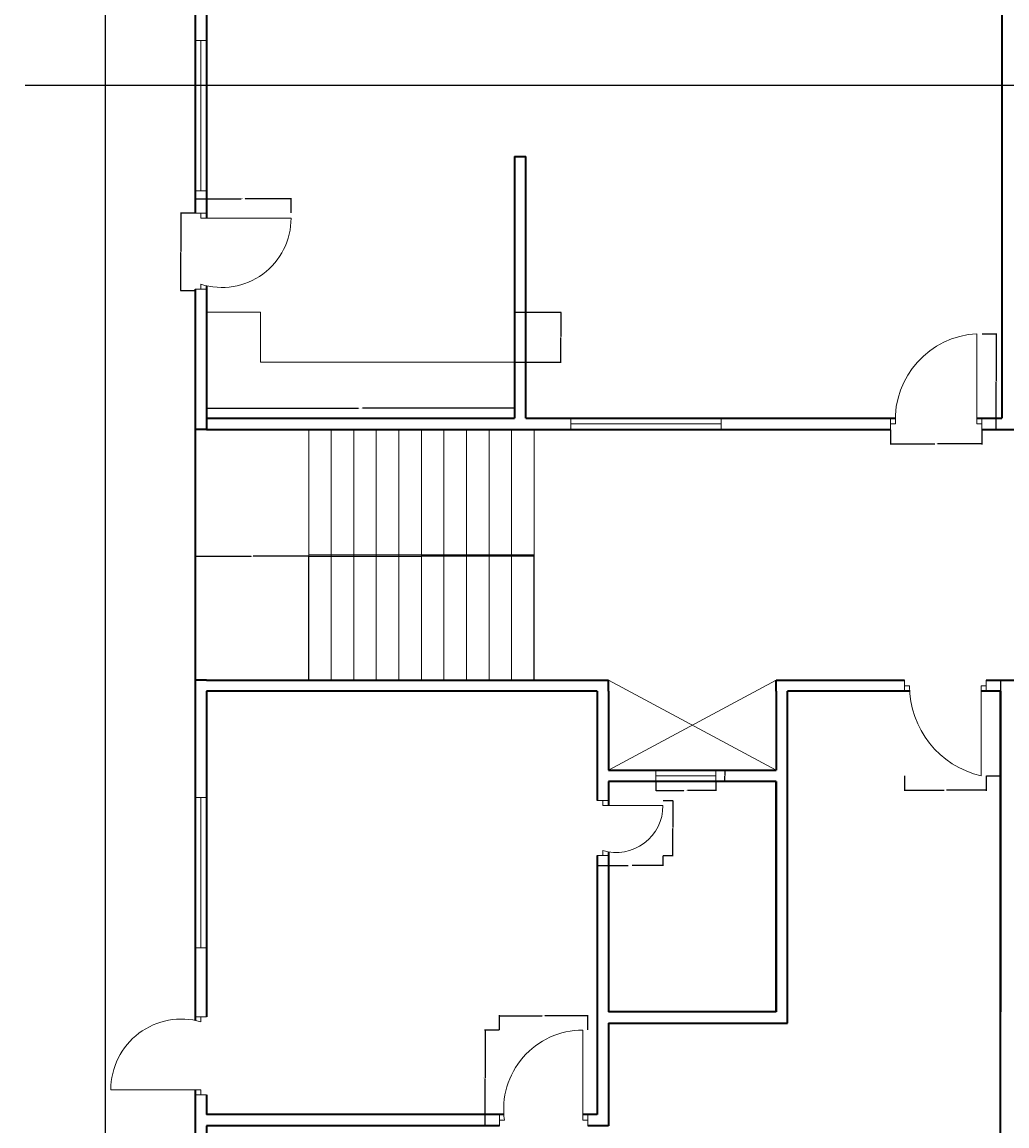
# Model space of a CAD drawing. Units: inches. Extents: x 1520 to 3401, y 1570 to 3432.
# Tile 11 of 15: x 2435 to 2828, y 2061 to 2501. Entities that reach past the tile are written whole.
import ezdxf

# ---------------------------------------------------------------- set-up
doc = ezdxf.new("R2010")
doc.units = ezdxf.units.IN
for name, color, linetype, lineweight in [('A-ANNO-DIMS', 2, 'Continuous', 18), ('A-ANNO-SYMB', 2, 'Continuous', 25), ('A-DOOR', 3, 'Continuous', 18), ('A-FLOR-CASE', 8, 'Continuous', 18), ('A-FLOR-EDGE', 7, 'Continuous', 25), ('A-FLOR-OPEN', 8, 'Continuous', 13), ('A-FLOR-STRS', 2, 'Continuous', 18), ('A-GLAZ', 4, 'Continuous', 18), ('A-WALL', 7, 'Continuous', 35)]:
    doc.layers.add(name, color=color, linetype=linetype, lineweight=lineweight)
doc.styles.get("Standard").update_dxf_attribs({"font": 'arial.ttf'})
doc.dimstyles.get("Standard").update_dxf_attribs({"dimtxt": 0.18, "dimasz": 0.18, "dimexe": 0.18, "dimexo": 0.0625, "dimgap": 0.09, "dimtad": 0, "dimtih": 1, "dimtoh": 1, "dimdec": 4, "dimzin": 0, "dimdsep": 46, "dimtxsty": 'Standard', "dimcen": 0.09, "dimadec": 0, "dimazin": 0, "dimtfac": 1, "dimtdec": 4, "dimtofl": 0, "dimtmove": 0, "dimatfit": 3, "dimfxl": 1, "dimtolj": 1, "dimtzin": 0, "dimarcsym": 0})

# ---------------------------------------------------------------- blocks, each defined once
blk = doc.blocks.new('DOOR-SWING-36-09')
for p, q in [((34.55, 2.25), (34.55, 38.25)), ((0, 4.5), (0, 0)), ((36.55, 4.5), (36.55, 0)), ((0, 0), (0, 2.25)), ((0, 2.25), (2, 2.25)), ((36.55, 2.25), (34.55, 2.25)), ((36.55, 0), (36.55, 2.25))]:
    blk.add_line(p, q)
blk.add_arc((36.37, 3.88), 34.41, 93.0408, 182.7237)
blk = doc.blocks.new('DOOR-SWING-24-14')
for p, q in [((4.5, 21.95), (0, 21.95)), ((0, 21.95), (2.25, 21.95)), ((2.25, 21.95), (2.25, 19.95)), ((2.25, 19.95), (26.25, 19.95)), ((4.5, 0), (0, 0)), ((0, 0), (2.25, 0)), ((2.25, 0), (2.25, 2))]:
    blk.add_line(p, q)
blk.add_arc((7.54, 19.95), 18.71, 253.5847, 0)
blk = doc.blocks.new('DOOR-SWING-36-15')
for p, q in [((33.3, 2.25), (33.3, 38.25)), ((0, 4.5), (0, 0)), ((35.3, 4.5), (35.3, 0)), ((0, 0), (0, 2.25)), ((0, 2.25), (2, 2.25)), ((35.3, 2.25), (33.3, 2.25)), ((35.3, 0), (35.3, 2.25))]:
    blk.add_line(p, q)
blk.add_arc((33.3, 6.65), 31.6, 90, 187.995)
blk = doc.blocks.new('DOOR-SWING-36-17')
for p, q in [((0, 33.75), (0, 38.25)), ((0, 38.25), (0, 36)), ((0, 36), (2, 36)), ((32.63, 36), (30.63, 36)), ((30.63, 36), (30.63, 0)), ((32.63, 33.75), (32.63, 38.25)), ((32.63, 38.25), (32.63, 36))]:
    blk.add_line(p, q)
blk.add_arc((38.95, 36), 36.95, 180, 256.9796)
blk = doc.blocks.new('DOOR-SWING-36-24')
for p, q in [((0, 30.42), (4.5, 30.42)), ((4.5, 30.42), (2.25, 30.42)), ((2.25, 30.42), (2.25, 28.42)), ((2.25, 28.42), (38.25, 28.42)), ((4.5, 0), (0, 0)), ((0, 0), (2.25, 0)), ((2.25, 0), (2.25, 2))]:
    blk.add_line(p, q)
blk.add_arc((10.55, 28.42), 27.7, 252.5577, 0)
blk = doc.blocks.new('DOOR-SWING-36-25')
for p, q in [((33.75, 31.15), (38.25, 31.15)), ((38.25, 31.15), (36, 31.15)), ((36, 31.15), (36, 29.15)), ((36, 2), (0, 2)), ((38.25, 0), (33.75, 0)), ((33.75, 0), (36, 0)), ((36, 0), (36, 2))]:
    blk.add_line(p, q)
blk.add_arc((28.23, 2), 28.23, 74.0345, 180)
blk = doc.blocks.new('WIN-PLAN-24-01')
for p, q in [((0, 4.5), (0, 0)), ((24, 2.25), (24, 4.5)), ((24, 4.5), (24, 0)), ((0, 0), (0, 2.25)), ((0, 2.25), (24, 2.25))]:
    blk.add_line(p, q)
blk = doc.blocks.new('WIN-PLAN-60-02')
for p, q in [((4.5, 60), (0, 60)), ((0, 60), (2.25, 60)), ((2.25, 60), (2.25, 0)), ((4.5, 0), (0, 0)), ((2.25, 0), (4.5, 0))]:
    blk.add_line(p, q)
blk = doc.blocks.new('WIN-PLAN-60-03')
for p, q in [((0, 2.25), (0, 4.5)), ((0, 4.5), (0, 0)), ((60, 0), (60, 4.5)), ((60, 4.5), (60, 2.25)), ((60, 2.25), (0, 2.25))]:
    blk.add_line(p, q)
blk = doc.blocks.new('KITCHEN-COUNTER-04')
for p, q in [((0, 19.94), (21.46, 19.94)), ((21.46, 19.94), (21.46, 0)), ((21.46, 0), (123, 0)), ((123, 0), (123, 0))]:
    blk.add_line(p, q)
blk = doc.blocks.new('*D63')
at = {"layer": 'A-ANNO-DIMS', "color": 0, "lineweight": -2, "transparency": 16777216}
for p, q in [((2687.73, 2198.12), (2687.73, 2194.4)), ((2687.91, 2194.58), (2698.98, 2194.58)), ((2711.55, 2194.58), (2700.49, 2194.58)), ((2711.73, 2198.12), (2711.73, 2194.4))]:
    blk.add_line(p, q, dxfattribs=at)
at = {"layer": 'A-ANNO-DIMS', "color": 0, "transparency": 16777216}
for points in [[(2687.91, 2194.61), (2687.91, 2194.55), (2687.73, 2194.58)], [(2711.55, 2194.61), (2711.55, 2194.55), (2711.73, 2194.58)]]:
    blk.add_solid(points, dxfattribs=at)
at = {"layer": 'Defpoints', "color": 0, "transparency": 16777216}
for p in [(2687.73, 2198.18), (2711.73, 2198.18), (2711.73, 2194.58)]:
    blk.add_point(p, dxfattribs=at)
at = {"layer": 'A-ANNO-DIMS', "color": 0, "transparency": 16777216, "insert": (2699.73, 2194.58), "char_height": 0.18, "attachment_point": 5}
blk.add_mtext('\\A1;W1 24 TYP.', dxfattribs=at)
blk = doc.blocks.new('*D64')
at = {"layer": 'A-ANNO-DIMS', "color": 0, "lineweight": -2, "transparency": 16777216}
for p, q in [((2711.79, 2202.68), (2715.51, 2202.68)), ((2715.33, 2202.5), (2715.33, 2200.61)), ((2715.33, 2198.36), (2715.33, 2200.25)), ((2711.79, 2198.18), (2715.51, 2198.18))]:
    blk.add_line(p, q, dxfattribs=at)
at = {"layer": 'A-ANNO-DIMS', "color": 0, "transparency": 16777216}
for points in [[(2715.3, 2202.5), (2715.36, 2202.5), (2715.33, 2202.68)], [(2715.3, 2198.36), (2715.36, 2198.36), (2715.33, 2198.18)]]:
    blk.add_solid(points, dxfattribs=at)
at = {"layer": 'Defpoints', "color": 0, "transparency": 16777216}
for p in [(2711.73, 2202.68), (2715.33, 2202.68), (2711.73, 2198.18)]:
    blk.add_point(p, dxfattribs=at)
at = {"layer": 'A-ANNO-DIMS', "color": 0, "transparency": 16777216, "insert": (2715.33, 2200.43), "char_height": 0.18, "attachment_point": 5}
blk.add_mtext('\\A1;5 TYP.', dxfattribs=at)
blk = doc.blocks.new('*D97')
at = {"layer": 'A-ANNO-DIMS', "color": 0, "lineweight": -2, "transparency": 16777216}
for p, q in [((2818.06, 2376.93), (2823.92, 2376.93)), ((2823.74, 2376.75), (2823.74, 2357.99)), ((2823.74, 2338.86), (2823.74, 2357.62)), ((2818.06, 2338.68), (2823.92, 2338.68))]:
    blk.add_line(p, q, dxfattribs=at)
at = {"layer": 'A-ANNO-DIMS', "color": 0, "transparency": 16777216}
for points in [[(2823.71, 2376.75), (2823.77, 2376.75), (2823.74, 2376.93)], [(2823.71, 2338.86), (2823.77, 2338.86), (2823.74, 2338.68)]]:
    blk.add_solid(points, dxfattribs=at)
at = {"layer": 'Defpoints', "color": 0, "transparency": 16777216}
for p in [(2818, 2376.93), (2823.74, 2376.93), (2818, 2338.68)]:
    blk.add_point(p, dxfattribs=at)
at = {"layer": 'A-ANNO-DIMS', "color": 0, "transparency": 16777216, "insert": (2823.74, 2357.8), "char_height": 0.18, "attachment_point": 5}
blk.add_mtext('\\A1;D09 38 TYP.', dxfattribs=at)
blk = doc.blocks.new('*D98')
at = {"layer": 'A-ANNO-DIMS', "color": 0, "lineweight": -2, "transparency": 16777216}
for p, q in [((2781.45, 2338.62), (2781.45, 2332.76)), ((2818, 2338.62), (2818, 2332.76)), ((2781.63, 2332.94), (2799.2, 2332.94)), ((2817.82, 2332.94), (2800.25, 2332.94))]:
    blk.add_line(p, q, dxfattribs=at)
at = {"layer": 'A-ANNO-DIMS', "color": 0, "transparency": 16777216}
for points in [[(2781.63, 2332.97), (2781.63, 2332.91), (2781.45, 2332.94)], [(2817.82, 2332.97), (2817.82, 2332.91), (2818, 2332.94)]]:
    blk.add_solid(points, dxfattribs=at)
at = {"layer": 'Defpoints', "color": 0, "transparency": 16777216}
for p in [(2781.45, 2338.68), (2818, 2338.68), (2818, 2332.94)]:
    blk.add_point(p, dxfattribs=at)
at = {"layer": 'A-ANNO-DIMS', "color": 0, "transparency": 16777216, "insert": (2799.72, 2332.94), "char_height": 0.18, "attachment_point": 5}
blk.add_mtext('\\A1;37 TYP.', dxfattribs=at)
blk = doc.blocks.new('*D107')
at = {"layer": 'A-ANNO-DIMS', "color": 0, "lineweight": -2, "transparency": 16777216}
for p, q in [((2664.4, 2168.53), (2664.4, 2164.47)), ((2690.65, 2168.53), (2690.65, 2164.47)), ((2664.58, 2164.65), (2676.73, 2164.65)), ((2690.47, 2164.65), (2678.31, 2164.65))]:
    blk.add_line(p, q, dxfattribs=at)
at = {"layer": 'A-ANNO-DIMS', "color": 0, "transparency": 16777216}
for points in [[(2664.58, 2164.68), (2664.58, 2164.62), (2664.4, 2164.65)], [(2690.47, 2164.68), (2690.47, 2164.62), (2690.65, 2164.65)]]:
    blk.add_solid(points, dxfattribs=at)
at = {"layer": 'Defpoints', "color": 0, "transparency": 16777216}
for p in [(2664.4, 2168.59), (2690.65, 2168.59), (2690.65, 2164.65)]:
    blk.add_point(p, dxfattribs=at)
at = {"layer": 'A-ANNO-DIMS', "color": 0, "transparency": 16777216, "insert": (2677.52, 2164.65), "char_height": 0.18, "attachment_point": 5}
blk.add_mtext('\\A1;D14 26 TYP.', dxfattribs=at)
blk = doc.blocks.new('*D108')
at = {"layer": 'A-ANNO-DIMS', "color": 0, "lineweight": -2, "transparency": 16777216}
for p, q in [((2690.71, 2190.54), (2694.77, 2190.54)), ((2694.59, 2190.36), (2694.59, 2179.75)), ((2694.59, 2168.77), (2694.59, 2179.39)), ((2690.71, 2168.59), (2694.77, 2168.59))]:
    blk.add_line(p, q, dxfattribs=at)
at = {"layer": 'A-ANNO-DIMS', "color": 0, "transparency": 16777216}
for points in [[(2694.56, 2190.36), (2694.62, 2190.36), (2694.59, 2190.54)], [(2694.56, 2168.77), (2694.62, 2168.77), (2694.59, 2168.59)]]:
    blk.add_solid(points, dxfattribs=at)
at = {"layer": 'Defpoints', "color": 0, "transparency": 16777216}
for p in [(2690.65, 2190.54), (2694.59, 2190.54), (2690.65, 2168.59)]:
    blk.add_point(p, dxfattribs=at)
at = {"layer": 'A-ANNO-DIMS', "color": 0, "transparency": 16777216, "insert": (2694.59, 2179.57), "char_height": 0.18, "attachment_point": 5}
blk.add_mtext('\\A1;22 TYP.', dxfattribs=at)
blk = doc.blocks.new('*D109')
at = {"layer": 'A-ANNO-DIMS', "color": 0, "lineweight": -2, "transparency": 16777216}
for p, q in [((2625.26, 2098.93), (2619.41, 2098.93)), ((2619.59, 2098.75), (2619.59, 2079.99)), ((2619.59, 2060.86), (2619.59, 2079.62)), ((2625.26, 2060.68), (2619.41, 2060.68))]:
    blk.add_line(p, q, dxfattribs=at)
at = {"layer": 'A-ANNO-DIMS', "color": 0, "transparency": 16777216}
for points in [[(2619.56, 2098.75), (2619.62, 2098.75), (2619.59, 2098.93)], [(2619.56, 2060.86), (2619.62, 2060.86), (2619.59, 2060.68)]]:
    blk.add_solid(points, dxfattribs=at)
at = {"layer": 'Defpoints', "color": 0, "transparency": 16777216}
for p in [(2619.59, 2098.93), (2625.32, 2098.93), (2625.32, 2060.68)]:
    blk.add_point(p, dxfattribs=at)
at = {"layer": 'A-ANNO-DIMS', "color": 0, "transparency": 16777216, "insert": (2619.59, 2079.8), "char_height": 0.18, "attachment_point": 5}
blk.add_mtext('\\A1;D15 38 TYP.', dxfattribs=at)
blk = doc.blocks.new('*D110')
at = {"layer": 'A-ANNO-DIMS', "color": 0, "lineweight": -2, "transparency": 16777216}
for p, q in [((2625.32, 2098.99), (2625.32, 2104.85)), ((2625.5, 2104.67), (2642.45, 2104.67)), ((2660.44, 2104.67), (2643.5, 2104.67)), ((2660.62, 2098.99), (2660.62, 2104.85))]:
    blk.add_line(p, q, dxfattribs=at)
at = {"layer": 'A-ANNO-DIMS', "color": 0, "transparency": 16777216}
for points in [[(2625.5, 2104.7), (2625.5, 2104.64), (2625.32, 2104.67)], [(2660.44, 2104.7), (2660.44, 2104.64), (2660.62, 2104.67)]]:
    blk.add_solid(points, dxfattribs=at)
at = {"layer": 'Defpoints', "color": 0, "transparency": 16777216}
for p in [(2660.62, 2104.67), (2625.32, 2098.93), (2660.62, 2098.93)]:
    blk.add_point(p, dxfattribs=at)
at = {"layer": 'A-ANNO-DIMS', "color": 0, "transparency": 16777216, "insert": (2642.97, 2104.67), "char_height": 0.18, "attachment_point": 5}
blk.add_mtext('\\A1;35 TYP.', dxfattribs=at)
blk = doc.blocks.new('*D113')
at = {"layer": 'A-ANNO-DIMS', "color": 0, "lineweight": -2, "transparency": 16777216}
for p, q in [((2819.78, 2238.68), (2825.63, 2238.68)), ((2825.45, 2238.5), (2825.45, 2219.74)), ((2825.45, 2200.61), (2825.45, 2219.37)), ((2819.78, 2200.43), (2825.63, 2200.43))]:
    blk.add_line(p, q, dxfattribs=at)
at = {"layer": 'A-ANNO-DIMS', "color": 0, "transparency": 16777216}
for points in [[(2825.42, 2238.5), (2825.48, 2238.5), (2825.45, 2238.68)], [(2825.42, 2200.61), (2825.48, 2200.61), (2825.45, 2200.43)]]:
    blk.add_solid(points, dxfattribs=at)
at = {"layer": 'Defpoints', "color": 0, "transparency": 16777216}
for p in [(2819.71, 2238.68), (2825.45, 2238.68), (2819.71, 2200.43)]:
    blk.add_point(p, dxfattribs=at)
at = {"layer": 'A-ANNO-DIMS', "color": 0, "transparency": 16777216, "insert": (2825.45, 2219.55), "char_height": 0.18, "attachment_point": 5}
blk.add_mtext('\\A1;D17 38 TYP.', dxfattribs=at)
blk = doc.blocks.new('*D114')
at = {"layer": 'A-ANNO-DIMS', "color": 0, "lineweight": -2, "transparency": 16777216}
for p, q in [((2787.09, 2200.37), (2787.09, 2194.51)), ((2819.71, 2200.37), (2819.71, 2194.51)), ((2787.27, 2194.69), (2802.87, 2194.69)), ((2819.53, 2194.69), (2803.93, 2194.69))]:
    blk.add_line(p, q, dxfattribs=at)
at = {"layer": 'A-ANNO-DIMS', "color": 0, "transparency": 16777216}
for points in [[(2787.27, 2194.72), (2787.27, 2194.66), (2787.09, 2194.69)], [(2819.53, 2194.72), (2819.53, 2194.66), (2819.71, 2194.69)]]:
    blk.add_solid(points, dxfattribs=at)
at = {"layer": 'Defpoints', "color": 0, "transparency": 16777216}
for p in [(2787.09, 2200.43), (2819.71, 2200.43), (2819.71, 2194.69)]:
    blk.add_point(p, dxfattribs=at)
at = {"layer": 'A-ANNO-DIMS', "color": 0, "transparency": 16777216, "insert": (2803.4, 2194.69), "char_height": 0.18, "attachment_point": 5}
blk.add_mtext('\\A1;33 TYP.', dxfattribs=at)
blk = doc.blocks.new('*D127')
at = {"layer": 'A-ANNO-DIMS', "color": 0, "lineweight": -2, "transparency": 16777216}
for p, q in [((2503.9, 2425.16), (2503.9, 2431.02)), ((2504.08, 2430.84), (2522.23, 2430.84)), ((2541.97, 2430.84), (2523.81, 2430.84)), ((2542.15, 2425.16), (2542.15, 2431.02))]:
    blk.add_line(p, q, dxfattribs=at)
at = {"layer": 'A-ANNO-DIMS', "color": 0, "transparency": 16777216}
for points in [[(2504.08, 2430.87), (2504.08, 2430.81), (2503.9, 2430.84)], [(2541.97, 2430.87), (2541.97, 2430.81), (2542.15, 2430.84)]]:
    blk.add_solid(points, dxfattribs=at)
at = {"layer": 'Defpoints', "color": 0, "transparency": 16777216}
for p in [(2542.15, 2430.84), (2503.9, 2425.1), (2542.15, 2425.1)]:
    blk.add_point(p, dxfattribs=at)
at = {"layer": 'A-ANNO-DIMS', "color": 0, "transparency": 16777216, "insert": (2523.02, 2430.84), "char_height": 0.18, "attachment_point": 5}
blk.add_mtext('\\A1;D24 38 TYP.', dxfattribs=at)
blk = doc.blocks.new('*D128')
at = {"layer": 'A-ANNO-DIMS', "color": 0, "lineweight": -2, "transparency": 16777216}
for p, q in [((2503.84, 2425.1), (2497.98, 2425.1)), ((2498.16, 2424.92), (2498.16, 2409.75)), ((2498.16, 2394.21), (2498.16, 2409.38)), ((2503.84, 2394.03), (2497.98, 2394.03))]:
    blk.add_line(p, q, dxfattribs=at)
at = {"layer": 'A-ANNO-DIMS', "color": 0, "transparency": 16777216}
for points in [[(2498.13, 2424.92), (2498.19, 2424.92), (2498.16, 2425.1)], [(2498.13, 2394.21), (2498.19, 2394.21), (2498.16, 2394.03)]]:
    blk.add_solid(points, dxfattribs=at)
at = {"layer": 'Defpoints', "color": 0, "transparency": 16777216}
for p in [(2498.16, 2425.1), (2503.9, 2425.1), (2503.9, 2394.03)]:
    blk.add_point(p, dxfattribs=at)
at = {"layer": 'A-ANNO-DIMS', "color": 0, "transparency": 16777216, "insert": (2498.16, 2409.56), "char_height": 0.18, "attachment_point": 5}
blk.add_mtext('\\A1;31 TYP.', dxfattribs=at)
blk = doc.blocks.new('*D155')
at = {"layer": 'A-ANNO-DIMS', "color": 0, "lineweight": -2, "transparency": 16777216}
for p, q in [((2508.4, 2365.57), (2508.4, 2347)), ((2631.4, 2365.57), (2631.4, 2347)), ((2508.58, 2347.18), (2569.11, 2347.18)), ((2631.22, 2347.18), (2570.69, 2347.18))]:
    blk.add_line(p, q, dxfattribs=at)
at = {"layer": 'A-ANNO-DIMS', "color": 0, "transparency": 16777216}
for points in [[(2508.58, 2347.21), (2508.58, 2347.15), (2508.4, 2347.18)], [(2631.22, 2347.21), (2631.22, 2347.15), (2631.4, 2347.18)]]:
    blk.add_solid(points, dxfattribs=at)
at = {"layer": 'Defpoints', "color": 0, "transparency": 16777216}
for p in [(2508.4, 2365.63), (2631.4, 2365.63), (2631.4, 2347.18)]:
    blk.add_point(p, dxfattribs=at)
at = {"layer": 'A-ANNO-DIMS', "color": 0, "transparency": 16777216, "insert": (2569.9, 2347.18), "char_height": 0.18, "attachment_point": 5}
blk.add_mtext('\\A1;C4 123 TYP.', dxfattribs=at)
blk = doc.blocks.new('*D156')
at = {"layer": 'A-ANNO-DIMS', "color": 0, "lineweight": -2, "transparency": 16777216}
for p, q in [((2631.46, 2385.57), (2650.03, 2385.57)), ((2649.85, 2385.39), (2649.85, 2375.78)), ((2649.85, 2365.81), (2649.85, 2375.42)), ((2631.46, 2365.63), (2650.03, 2365.63))]:
    blk.add_line(p, q, dxfattribs=at)
at = {"layer": 'A-ANNO-DIMS', "color": 0, "transparency": 16777216}
for points in [[(2649.82, 2385.39), (2649.88, 2385.39), (2649.85, 2385.57)], [(2649.82, 2365.81), (2649.88, 2365.81), (2649.85, 2365.63)]]:
    blk.add_solid(points, dxfattribs=at)
at = {"layer": 'Defpoints', "color": 0, "transparency": 16777216}
for p in [(2631.4, 2385.57), (2649.85, 2385.57), (2631.4, 2365.63)]:
    blk.add_point(p, dxfattribs=at)
at = {"layer": 'A-ANNO-DIMS', "color": 0, "transparency": 16777216, "insert": (2649.85, 2375.6), "char_height": 0.18, "attachment_point": 5}
blk.add_mtext('\\A1;20 TYP.', dxfattribs=at)
blk = doc.blocks.new('*D192')
at = {"layer": 'A-ANNO-DIMS', "color": 0, "lineweight": -2, "transparency": 16777216}
for p, q in [((2467.84, 2733.18), (2386.32, 2733.18)), ((2386.5, 2733), (2386.5, 2244.61)), ((2386.5, 1755.86), (2386.5, 2244.25)), ((2503.84, 1755.68), (2386.32, 1755.68))]:
    blk.add_line(p, q, dxfattribs=at)
at = {"layer": 'A-ANNO-DIMS', "color": 0, "transparency": 16777216}
for points in [[(2386.47, 2733), (2386.53, 2733), (2386.5, 2733.18)], [(2386.47, 1755.86), (2386.53, 1755.86), (2386.5, 1755.68)]]:
    blk.add_solid(points, dxfattribs=at)
at = {"layer": 'Defpoints', "color": 0, "transparency": 16777216}
for p in [(2467.9, 2733.18), (2386.5, 1755.68), (2503.9, 1755.68)]:
    blk.add_point(p, dxfattribs=at)
at = {"layer": 'A-ANNO-DIMS', "color": 0, "transparency": 16777216, "insert": (2386.5, 2244.43), "char_height": 0.18, "attachment_point": 5}
blk.add_mtext('\\A1;977.5', dxfattribs=at)
blk = doc.blocks.new('*D207')
at = {"layer": 'A-ANNO-DIMS', "color": 0, "lineweight": -2, "transparency": 16777216}
for p, q in [((2549.18, 2238.74), (2549.18, 2288.26)), ((2549.36, 2288.08), (2593.96, 2288.08)), ((2639, 2288.08), (2594.4, 2288.08)), ((2639.18, 2238.74), (2639.18, 2288.26))]:
    blk.add_line(p, q, dxfattribs=at)
at = {"layer": 'A-ANNO-DIMS', "color": 0, "transparency": 16777216}
for points in [[(2549.36, 2288.11), (2549.36, 2288.05), (2549.18, 2288.08)], [(2639, 2288.11), (2639, 2288.05), (2639.18, 2288.08)]]:
    blk.add_solid(points, dxfattribs=at)
at = {"layer": 'Defpoints', "color": 0, "transparency": 16777216}
for p in [(2639.18, 2288.08), (2549.18, 2238.68), (2639.18, 2238.68)]:
    blk.add_point(p, dxfattribs=at)
at = {"layer": 'A-ANNO-DIMS', "color": 0, "transparency": 16777216, "insert": (2594.18, 2288.08), "char_height": 0.18, "attachment_point": 5}
blk.add_mtext('\\A1;90', dxfattribs=at)
blk = doc.blocks.new('*D208')
at = {"layer": 'A-ANNO-DIMS', "color": 0, "lineweight": -2, "transparency": 16777216}
for p, q in [((2503.9, 2238.74), (2503.9, 2288.26)), ((2504.08, 2288.08), (2526.14, 2288.08)), ((2549, 2288.08), (2526.94, 2288.08)), ((2549.18, 2238.74), (2549.18, 2288.26))]:
    blk.add_line(p, q, dxfattribs=at)
at = {"layer": 'A-ANNO-DIMS', "color": 0, "transparency": 16777216}
for points in [[(2504.08, 2288.11), (2504.08, 2288.05), (2503.9, 2288.08)], [(2549, 2288.11), (2549, 2288.05), (2549.18, 2288.08)]]:
    blk.add_solid(points, dxfattribs=at)
at = {"layer": 'Defpoints', "color": 0, "transparency": 16777216}
for p in [(2549.18, 2288.08), (2503.9, 2238.68), (2549.18, 2238.68)]:
    blk.add_point(p, dxfattribs=at)
at = {"layer": 'A-ANNO-DIMS', "color": 0, "transparency": 16777216, "insert": (2526.54, 2288.08), "char_height": 0.18, "attachment_point": 5}
blk.add_mtext('\\A1;45.28', dxfattribs=at)

msp = doc.modelspace()

# ---------------------------------------------------------------- linework, layer by layer
at = {"layer": 'A-ANNO-SYMB'}
msp.add_line((2435.8982, 2476.123), (3251.5148, 2476.123), dxfattribs=at)
at = {"layer": 'A-FLOR-EDGE'}
msp.add_line((2467.8987, 2733.1786), (2467.8987, 1791.6786), dxfattribs=at)
at = {"layer": 'A-FLOR-OPEN'}
for p, q in [((2735.8987, 2238.6786), (2668.8987, 2202.6786)), ((2668.8987, 2238.6786), (2735.8987, 2202.6786))]:
    msp.add_line(p, q, dxfattribs=at)
at = {"layer": 'A-FLOR-STRS'}
for p, q in [((2549.1766, 2238.6786), (2549.1766, 2338.6786)), ((2549.1766, 2338.6786), (2549.1766, 2288.6786)), ((2558.1766, 2238.6786), (2558.1766, 2338.6786)), ((2558.1766, 2338.6786), (2558.1766, 2288.6786)), ((2567.1766, 2238.6786), (2567.1766, 2338.6786)), ((2567.1766, 2338.6786), (2567.1766, 2288.6786)), ((2576.1766, 2238.6786), (2576.1766, 2338.6786)), ((2576.1766, 2338.6786), (2576.1766, 2288.6786)), ((2585.1766, 2238.6786), (2585.1766, 2338.6786)), ((2585.1766, 2338.6786), (2585.1766, 2288.6786)), ((2594.1766, 2238.6786), (2594.1766, 2338.6786)), ((2594.1766, 2338.6786), (2594.1766, 2288.6786)), ((2603.1766, 2238.6786), (2603.1766, 2338.6786)), ((2603.1766, 2338.6786), (2603.1766, 2288.6786)), ((2612.1766, 2238.6786), (2612.1766, 2338.6786)), ((2612.1766, 2338.6786), (2612.1766, 2288.6786)), ((2621.1766, 2238.6786), (2621.1766, 2338.6786)), ((2621.1766, 2338.6786), (2621.1766, 2288.6786)), ((2630.1766, 2238.6786), (2630.1766, 2338.6786)), ((2630.1766, 2338.6786), (2630.1766, 2288.6786)), ((2639.1766, 2238.6786), (2639.1766, 2338.6786)), ((2549.1766, 2288.6786), (2639.1766, 2288.6786))]:
    msp.add_line(p, q, dxfattribs=at)
at = {"layer": 'A-WALL'}
for p, q in [((2825.8987, 2558.1786), (2825.8987, 2343.1786)), ((2503.8987, 2508.6786), (2503.8987, 2425.0977)), ((2503.8987, 2508.6786), (2503.8987, 2425.0977)), ((2508.3987, 2508.6786), (2508.3987, 2423.0977)), ((2631.3987, 2447.697), (2631.3987, 2343.1786)), ((2631.3987, 2447.697), (2635.8987, 2447.697)), ((2635.8987, 2343.1786), (2635.8987, 2447.697)), ((2503.8987, 2394.6735), (2503.8987, 2102.8094)), ((2503.8987, 2394.6735), (2503.8987, 2102.8094)), ((2508.3987, 2396.0692), (2508.3987, 2338.6786)), ((2508.3987, 2343.1786), (2631.3987, 2343.1786)), ((2635.8987, 2343.1786), (2783.4164, 2343.1786)), ((2815.9986, 2343.1786), (2825.8987, 2343.1786)), ((2508.3987, 2338.6786), (2503.8987, 2338.6786)), ((2508.3987, 2338.6786), (2781.4498, 2338.6786)), ((2817.9986, 2338.6786), (2967.3389, 2338.6786)), ((2508.3987, 2238.6786), (2503.8987, 2238.6786)), ((2508.3987, 2238.6786), (2668.8987, 2238.6786)), ((2668.8987, 2234.1786), (2668.8987, 2238.6786)), ((2735.8987, 2238.6786), (2787.088, 2238.6786)), ((2735.8987, 2234.1786), (2735.8987, 2238.6786)), ((2819.7132, 2238.6786), (3032.072, 2238.6786)), ((2508.3987, 2234.1786), (2508.3987, 2104.2644)), ((2664.3987, 2234.1786), (2508.3987, 2234.1786)), ((2664.3987, 2234.1786), (2664.3987, 2190.5406)), ((2668.8987, 2234.1786), (2668.8987, 2202.6786)), ((2735.8987, 2234.1786), (2735.8987, 2202.6786)), ((2789.1566, 2234.1786), (2740.3987, 2234.1786)), ((2740.3987, 2106.1786), (2740.3987, 2234.1786)), ((2825.3987, 2234.1786), (2817.7132, 2234.1786)), ((2825.3987, 1923.6786), (2825.3987, 2234.1786)), ((2825.3987, 2234.1786), (2825.3987, 2106.1786)), ((2668.8987, 2202.6786), (2735.8987, 2202.6786)), ((2668.8987, 2198.1786), (2668.8987, 2188.5406)), ((2735.8987, 2198.1786), (2668.8987, 2198.1786)), ((2735.8987, 2198.1786), (2735.8987, 2106.1786)), ((2735.8987, 2106.1786), (2735.8987, 2198.1786)), ((2664.3987, 2168.5913), (2664.3987, 2065.1786)), ((2668.8987, 2170.0769), (2668.8987, 2106.1786)), ((2735.8987, 2106.1786), (2668.8987, 2106.1786)), ((2740.3987, 2101.6786), (2740.3987, 2106.1786)), ((2668.8987, 2101.6786), (2668.8987, 2060.6786)), ((2668.8987, 2101.6786), (2740.3987, 2101.6786)), ((2503.8987, 2075.1195), (2503.8987, 1924.1968)), ((2503.8987, 2075.1195), (2503.8987, 1924.1968)), ((2508.3987, 2073.1195), (2508.3987, 2065.1786)), ((2627.0907, 2065.1786), (2508.3987, 2065.1786)), ((2664.3987, 2065.1786), (2658.622, 2065.1786)), ((2508.3987, 2060.6786), (2508.3987, 1922.1968)), ((2625.3249, 2060.6786), (2508.3987, 2060.6786)), ((2668.8987, 2060.6786), (2660.622, 2060.6786))]:
    msp.add_line(p, q, dxfattribs=at)

# ---------------------------------------------------------------- block references
at = {"layer": 'A-DOOR'}
for name, p in [('DOOR-SWING-36-24', (2503.8988, 2394.673)), ('DOOR-SWING-36-09', (2781.4498, 2338.679)), ('DOOR-SWING-36-17', (2787.0878, 2200.429)), ('DOOR-SWING-24-14', (2664.3988, 2168.591)), ('DOOR-SWING-36-25', (2470.1488, 2073.119)), ('DOOR-SWING-36-15', (2625.3248, 2060.679))]:
    msp.add_blockref(name, p, dxfattribs=at)
at = {"layer": 'A-FLOR-CASE'}
msp.add_blockref('KITCHEN-COUNTER-04', (2508.3988, 2365.63), dxfattribs=at)
at = {"layer": 'A-GLAZ', "extrusion": (0, 0, -1), "zscale": -1, "rotation": 90}
msp.add_blockref('WIN-PLAN-60-03', (-2503.899, 2434.0305), dxfattribs=at)
at = {"layer": 'A-GLAZ'}
for name, p, rotation in [('WIN-PLAN-60-02', (2653.8695, 2343.1785), 270), ('WIN-PLAN-60-03', (2508.3983, 2131.8338), 90)]:
    msp.add_blockref(name, p, dxfattribs=dict(at, rotation=rotation))
msp.add_blockref('WIN-PLAN-24-01', (2687.7318, 2198.179), dxfattribs=at)

# ---------------------------------------------------------------- dimensions: what is measured, and where the dimension line sits
at = {"layer": 'A-ANNO-DIMS'}
dim = msp.add_linear_dim(base=(2386.4982, 1755.6786), p1=(2467.8987, 2733.1786), p2=(2503.8987, 1755.6786), angle=90, dimstyle='Standard', override={"dimdec": 1, "dimlfac": 1, "dimrnd": 0, "dimzin": 0, "dimdsep": 46, "dimlunit": 2}, dxfattribs=at)
dim.commit()
dim.dimension.update_dxf_attribs({"geometry": '*D192', "text_midpoint": (2386.4982, 2244.4286)})
for base, p1, p2, text, picture, middle in [((2542.1487, 2430.8352), (2503.8987, 2425.0977), (2542.1487, 2425.0977), 'D24 <> TYP.', '*D127', (2523.0237, 2430.8352)), ((2631.3987, 2347.1795), (2508.3987, 2365.6295), (2631.3987, 2365.6295), 'C4 <> TYP.', '*D155', (2569.8987, 2347.1795)), ((2817.9986, 2332.9411), (2781.4498, 2338.6786), (2817.9986, 2338.6786), '<> TYP.', '*D98', (2799.7242, 2332.9411)), ((2819.7132, 2194.6911), (2787.088, 2200.4286), (2819.7132, 2200.4286), '<> TYP.', '*D114', (2803.4006, 2194.6911)), ((2711.7322, 2194.5786), (2687.7322, 2198.1786), (2711.7322, 2198.1786), 'W1 <> TYP.', '*D63', (2699.7322, 2194.5786)), ((2690.6487, 2164.6538), (2664.3987, 2168.5913), (2690.6487, 2168.5913), 'D14 <> TYP.', '*D107', (2677.5237, 2164.6538)), ((2660.622, 2104.6661), (2625.3249, 2098.9286), (2660.622, 2098.9286), '<> TYP.', '*D110', (2642.9735, 2104.6661))]:
    dim = msp.add_linear_dim(base=base, p1=p1, p2=p2, text=text, dimstyle='Standard', override={"dimdec": 0, "dimlfac": 1, "dimrnd": 0, "dimzin": 0, "dimdsep": 46, "dimlunit": 2}, dxfattribs=at)
    dim.commit()
    dim.dimension.update_dxf_attribs({"geometry": picture, "text_midpoint": middle})
for base, p1, p2, text, picture, middle in [((2498.1612, 2425.0977), (2503.8987, 2394.0301), (2503.8987, 2425.0977), '<> TYP.', '*D128', (2498.1612, 2409.5639)), ((2649.8487, 2385.5713), (2631.3987, 2365.6295), (2631.3987, 2385.5713), '<> TYP.', '*D156', (2649.8487, 2375.6004)), ((2823.7361, 2376.9286), (2817.9986, 2338.6786), (2817.9986, 2376.9286), 'D09 <> TYP.', '*D97', (2823.7361, 2357.8036)), ((2825.4507, 2238.6786), (2819.7132, 2200.4286), (2819.7132, 2238.6786), 'D17 <> TYP.', '*D113', (2825.4507, 2219.5536)), ((2715.3321503742, 2202.6786294992), (2711.7321503742, 2198.1786294992), (2711.7321503742, 2202.6786294992), '<> TYP.', '*D64', (2715.3321503742, 2200.4286294992)), ((2694.5862, 2190.5406), (2690.6487, 2168.5913), (2690.6487, 2190.5406), '<> TYP.', '*D108', (2694.5862, 2179.566)), ((2619.5874, 2098.9286), (2625.3249, 2060.6786), (2625.3249, 2098.9286), 'D15 <> TYP.', '*D109', (2619.5874, 2079.8036))]:
    dim = msp.add_linear_dim(base=base, p1=p1, p2=p2, angle=90, text=text, dimstyle='Standard', override={"dimdec": 0, "dimlfac": 1, "dimrnd": 0, "dimzin": 0, "dimdsep": 46, "dimlunit": 2}, dxfattribs=at)
    dim.commit()
    dim.dimension.update_dxf_attribs({"geometry": picture, "text_midpoint": middle})
for base, p1, p2, override, picture, middle in [((2549.1766, 2288.0786), (2503.8987, 2238.6786), (2549.1766, 2238.6786), {"dimdec": 2, "dimlfac": 1, "dimrnd": 0, "dimzin": 0, "dimdsep": 46, "dimlunit": 2}, '*D208', (2526.5376, 2288.0786)), ((2639.1766, 2288.0786), (2549.1766, 2238.6786), (2639.1766, 2238.6786), {"dimdec": 0, "dimlfac": 1, "dimrnd": 0, "dimzin": 0, "dimdsep": 46, "dimlunit": 2}, '*D207', (2594.1766, 2288.0786))]:
    dim = msp.add_linear_dim(base=base, p1=p1, p2=p2, dimstyle='Standard', override=override, dxfattribs=at)
    dim.commit()
    dim.dimension.update_dxf_attribs({"geometry": picture, "text_midpoint": middle})

doc.saveas('drawing.dxf')
